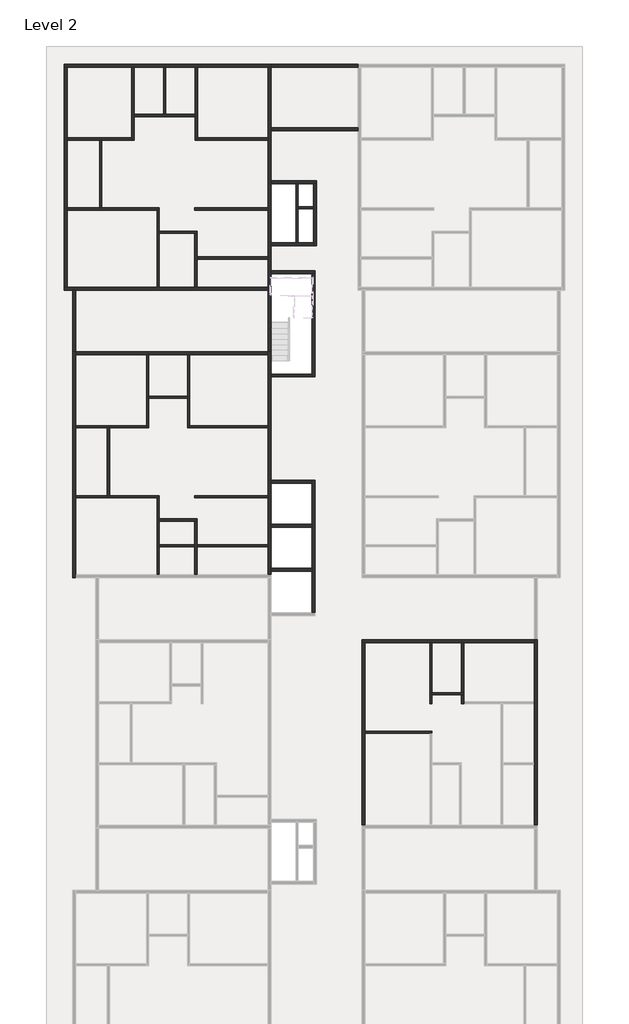
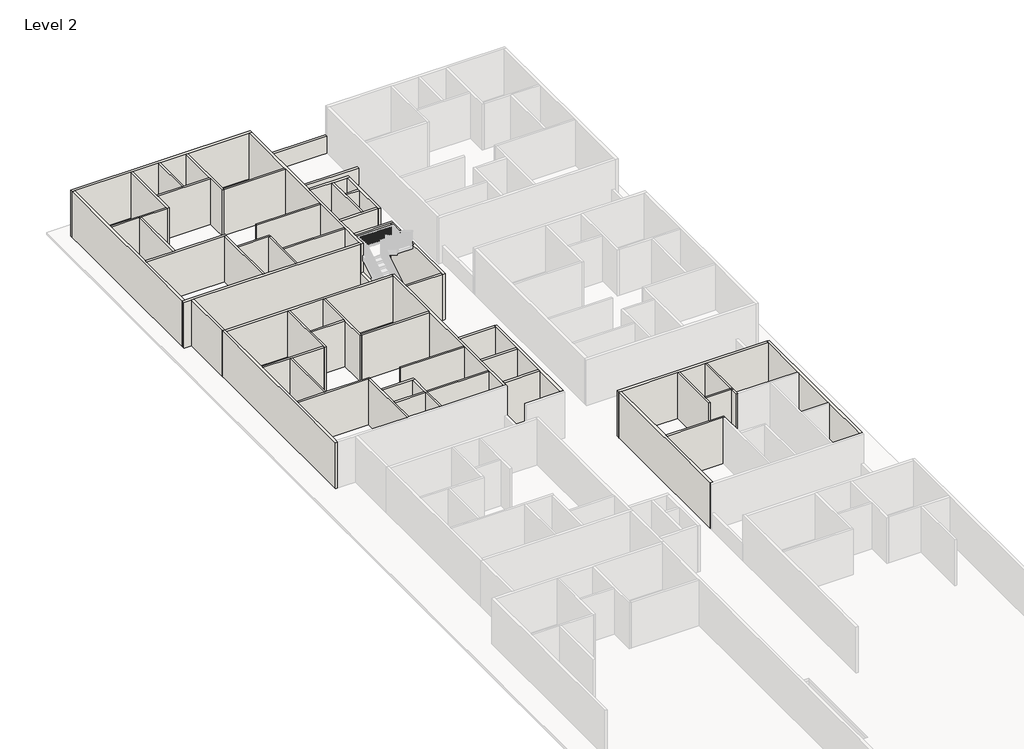
# One storey, part 3 of 8: 57 walls.
"""IFC4 building model written with IfcOpenShell, lengths in millimetres."""

from ifc_helpers import new_model, si_unit, frame, origin, place, context, project, spatial, polyline, outline, extrude, faceted_brep, element, save

model = new_model("IFC4")

# Units and contexts
model_context = context("Model", 3, world=origin())
ifc_project = project(units=[si_unit("LENGTHUNIT", "METRE", prefix="MILLI")], contexts=[model_context])

# Site, building, storey
site = spatial("IfcSite", under=ifc_project)
building = spatial("IfcBuilding", under=site)
storey = spatial("IfcBuildingStorey", under=building, Name="Level 2", Elevation=28282.6172466)

# Walls
placement = place(None, origin())
element("IfcWall", 1, ObjectType="4.5\"", at=placement, inside=storey, context=model_context, shape_type="Brep", body=[
    faceted_brep([(-10818.3415084, 35031.1216096, 28282.6172466), (-10818.3415084, 31373.5216096, 28282.6172466), (-10818.3415084, 31259.2216096, 28282.6172466), (-10818.3415084, 31259.2216096, 31330.6172466), (-10818.3415084, 31373.5216096, 31330.6172466), (-10818.3415084, 35031.1216096, 31330.6172466), (-10704.0415084, 35031.1216096, 28282.6172466), (-10704.0415084, 35031.1216096, 31330.6172466), (-10704.0415084, 32592.7216096, 31330.6172466), (-10704.0415084, 32478.4216096, 31330.6172466), (-10704.0415084, 31259.2216096, 31330.6172466), (-10704.0415084, 31259.2216096, 28282.6172466), (-10704.0415084, 32478.4216096, 28282.6172466), (-10704.0415084, 32592.7216096, 28282.6172466)], [[[0, 1, 2, 3, 4, 5]], [[6, 7, 8, 9, 10, 11, 12, 13]], [[2, 1, 0, 6, 13, 12, 11]], [[0, 5, 7, 6]], [[3, 2, 11, 10]], [[5, 4, 3, 10, 9, 8, 7]]]),
])
element("IfcWall", 2, ObjectType="4.5\"", at=placement, inside=storey, context=model_context, shape_type="Brep", body=[
    faceted_brep([(-10818.3415084, 31373.5216096, 28282.6172466), (-14171.1415084, 31373.5216096, 28282.6172466), (-14171.1415084, 31373.5216096, 31330.6172466), (-10818.3415084, 31373.5216096, 31330.6172466), (-10818.3415084, 31259.2216096, 28282.6172466), (-10818.3415084, 31259.2216096, 31330.6172466), (-12380.4415084, 31259.2216096, 31330.6172466), (-12494.7415084, 31259.2216096, 31330.6172466), (-14171.1415084, 31259.2216096, 31330.6172466), (-14171.1415084, 31259.2216096, 28282.6172466), (-12494.7415084, 31259.2216096, 28282.6172466), (-12380.4415084, 31259.2216096, 28282.6172466)], [[[0, 1, 2, 3]], [[4, 5, 6, 7, 8, 9, 10, 11]], [[1, 0, 4, 11, 10, 9]], [[0, 3, 5, 4]], [[2, 1, 9, 8]], [[3, 2, 8, 7, 6, 5]]]),
])
element("IfcWall", 3, ObjectType="4.5\"", at=placement, inside=storey, context=model_context, shape_type="SweptSolid", body=[
    extrude(outline(polyline([(-12494.7415084, 27754.0216096), (-12494.7415084, 31259.2216096), (-12380.4415084, 31259.2216096), (-12380.4415084, 27754.0216096), (-12494.7415084, 27754.0216096)])), frame((0.0, 0.0, 28282.6172466), z_axis=(0.0, 0.0, 1.0), x_axis=(1.0, 0.0, 0.0)), (0.0, 0.0, 1.0), 3048.0),
])
element("IfcWall", 4, ObjectType="4.5\"", at=placement, inside=storey, context=model_context, shape_type="Brep", body=[
    faceted_brep([(-14171.1415084, 27639.7216096, 28282.6172466), (-9510.2415084, 27639.7216096, 28282.6172466), (-9395.9415084, 27639.7216096, 28282.6172466), (-9395.9415084, 27639.7216096, 31330.6172466), (-9510.2415084, 27639.7216096, 31330.6172466), (-14171.1415084, 27639.7216096, 31330.6172466), (-14171.1415084, 27754.0216096, 28282.6172466), (-14171.1415084, 27754.0216096, 31330.6172466), (-12494.7415084, 27754.0216096, 31330.6172466), (-12380.4415084, 27754.0216096, 31330.6172466), (-9395.9415084, 27754.0216096, 31330.6172466), (-9395.9415084, 27754.0216096, 28282.6172466), (-12380.4415084, 27754.0216096, 28282.6172466), (-12494.7415084, 27754.0216096, 28282.6172466)], [[[0, 1, 2, 3, 4, 5]], [[6, 7, 8, 9, 10, 11, 12, 13]], [[2, 1, 0, 6, 13, 12, 11]], [[0, 5, 7, 6]], [[3, 2, 11, 10]], [[5, 4, 3, 10, 9, 8, 7]]]),
])
element("IfcWall", 5, ObjectType="4.5\"", at=placement, inside=storey, context=model_context, shape_type="Brep", body=[
    faceted_brep([(-9510.2415084, 27639.7216096, 28282.6172466), (-9510.2415084, 23651.9216096, 28282.6172466), (-9510.2415084, 23651.9216096, 31330.6172466), (-9510.2415084, 27639.7216096, 31330.6172466), (-9395.9415084, 27639.7216096, 28282.6172466), (-9395.9415084, 27639.7216096, 31330.6172466), (-9395.9415084, 26547.5216096, 31330.6172466), (-9395.9415084, 26433.2216096, 31330.6172466), (-9395.9415084, 23651.9216096, 31330.6172466), (-9395.9415084, 23651.9216096, 28282.6172466), (-9395.9415084, 26433.2216096, 28282.6172466), (-9395.9415084, 26547.5216096, 28282.6172466)], [[[0, 1, 2, 3]], [[4, 5, 6, 7, 8, 9, 10, 11]], [[1, 0, 4, 11, 10, 9]], [[0, 3, 5, 4]], [[2, 1, 9, 8]], [[3, 2, 8, 7, 6, 5]]]),
])
element("IfcWall", 6, ObjectType="4.5\"", at=placement, inside=storey, context=model_context, shape_type="Brep", body=[
    faceted_brep([(-9395.9415084, 26433.2216096, 28282.6172466), (-7567.1415084, 26433.2216096, 28282.6172466), (-7452.8415084, 26433.2216096, 28282.6172466), (-7452.8415084, 26433.2216096, 31330.6172466), (-7567.1415084, 26433.2216096, 31330.6172466), (-9395.9415084, 26433.2216096, 31330.6172466), (-9395.9415084, 26547.5216096, 28282.6172466), (-9395.9415084, 26547.5216096, 31330.6172466), (-7452.8415084, 26547.5216096, 31330.6172466), (-7452.8415084, 26547.5216096, 28282.6172466)], [[[0, 1, 2, 3, 4, 5]], [[6, 7, 8, 9]], [[2, 1, 0, 6, 9]], [[0, 5, 7, 6]], [[3, 2, 9, 8]], [[5, 4, 3, 8, 7]]]),
])
element("IfcWall", 7, ObjectType="4.5\"", at=placement, inside=storey, context=model_context, shape_type="Brep", body=[
    faceted_brep([(-7567.1415084, 26433.2216096, 28282.6172466), (-7567.1415084, 23651.9216096, 28282.6172466), (-7567.1415084, 23651.9216096, 31330.6172466), (-7567.1415084, 26433.2216096, 31330.6172466), (-7452.8415084, 26433.2216096, 28282.6172466), (-7452.8415084, 26433.2216096, 31330.6172466), (-7452.8415084, 25214.0216096, 31330.6172466), (-7452.8415084, 25099.7216096, 31330.6172466), (-7452.8415084, 23651.9216096, 31330.6172466), (-7452.8415084, 23651.9216096, 28282.6172466), (-7452.8415084, 25099.7216096, 28282.6172466), (-7452.8415084, 25214.0216096, 28282.6172466)], [[[0, 1, 2, 3]], [[4, 5, 6, 7, 8, 9, 10, 11]], [[1, 0, 4, 11, 10, 9]], [[0, 3, 5, 4]], [[2, 1, 9, 8]], [[3, 2, 8, 7, 6, 5]]]),
])
element("IfcWall", 8, ObjectType="4.5\"", at=placement, inside=storey, context=model_context, shape_type="SweptSolid", body=[
    extrude(outline(polyline([(-7452.8415084, 25214.0216096), (-3769.8415084, 25214.0216096), (-3769.8415084, 25099.7216096), (-7452.8415084, 25099.7216096), (-7452.8415084, 25214.0216096)])), frame((0.0, 0.0, 28282.6172466), z_axis=(0.0, 0.0, 1.0), x_axis=(1.0, 0.0, 0.0)), (0.0, 0.0, 1.0), 3048.0),
])
element("IfcWall", 9, ObjectType="4.5\"", at=placement, inside=storey, context=model_context, shape_type="SweptSolid", body=[
    extrude(outline(polyline([(-3769.8415084, 27639.7216096), (-7567.1415084, 27639.7216096), (-7567.1415084, 27754.0216096), (-3769.8415084, 27754.0216096), (-3769.8415084, 27639.7216096)])), frame((0.0, 0.0, 28282.6172466), z_axis=(0.0, 0.0, 1.0), x_axis=(1.0, 0.0, 0.0)), (0.0, 0.0, 1.0), 3048.0),
])
element("IfcWall", 10, ObjectType="4.5\"", at=placement, inside=storey, context=model_context, shape_type="Brep", body=[
    faceted_brep([(-10704.0415084, 32478.4216096, 28282.6172466), (-7541.7415084, 32478.4216096, 28282.6172466), (-7541.7415084, 32478.4216096, 31330.6172466), (-10704.0415084, 32478.4216096, 31330.6172466), (-10704.0415084, 32592.7216096, 28282.6172466), (-10704.0415084, 32592.7216096, 31330.6172466), (-9180.0415084, 32592.7216096, 31330.6172466), (-9065.7415084, 32592.7216096, 31330.6172466), (-7541.7415084, 32592.7216096, 31330.6172466), (-7541.7415084, 32592.7216096, 28282.6172466), (-9065.7415084, 32592.7216096, 28282.6172466), (-9180.0415084, 32592.7216096, 28282.6172466)], [[[0, 1, 2, 3]], [[4, 5, 6, 7, 8, 9, 10, 11]], [[1, 0, 4, 11, 10, 9]], [[0, 3, 5, 4]], [[2, 1, 9, 8]], [[3, 2, 8, 7, 6, 5]]]),
])
element("IfcWall", 11, ObjectType="4.5\"", at=placement, inside=storey, context=model_context, shape_type="SweptSolid", body=[
    extrude(outline(polyline([(-9180.0415084, 32592.7216096), (-9180.0415084, 35031.1216096), (-9065.7415084, 35031.1216096), (-9065.7415084, 32592.7216096), (-9180.0415084, 32592.7216096)])), frame((0.0, 0.0, 28282.6172466), z_axis=(0.0, 0.0, 1.0), x_axis=(1.0, 0.0, 0.0)), (0.0, 0.0, 1.0), 3048.0),
])
element("IfcWall", 12, ObjectType="4.5\"", at=placement, inside=storey, context=model_context, shape_type="Brep", body=[
    faceted_brep([(-7541.7415084, 35031.1216096, 28282.6172466), (-7541.7415084, 32592.7216096, 28282.6172466), (-7541.7415084, 32478.4216096, 28282.6172466), (-7541.7415084, 31259.2216096, 28282.6172466), (-7541.7415084, 31259.2216096, 31330.6172466), (-7541.7415084, 32478.4216096, 31330.6172466), (-7541.7415084, 32592.7216096, 31330.6172466), (-7541.7415084, 35031.1216096, 31330.6172466), (-7427.4415084, 35031.1216096, 28282.6172466), (-7427.4415084, 35031.1216096, 31330.6172466), (-7427.4415084, 31373.5216096, 31330.6172466), (-7427.4415084, 31259.2216096, 31330.6172466), (-7427.4415084, 31259.2216096, 28282.6172466), (-7427.4415084, 31373.5216096, 28282.6172466)], [[[0, 1, 2, 3, 4, 5, 6, 7]], [[8, 9, 10, 11, 12, 13]], [[3, 2, 1, 0, 8, 13, 12]], [[0, 7, 9, 8]], [[4, 3, 12, 11]], [[7, 6, 5, 4, 11, 10, 9]]]),
])
element("IfcWall", 13, ObjectType="4.5\"", at=placement, inside=storey, context=model_context, shape_type="SweptSolid", body=[
    extrude(outline(polyline([(-3769.8415084, 31259.2216096), (-7427.4415084, 31259.2216096), (-7427.4415084, 31373.5216096), (-3769.8415084, 31373.5216096), (-3769.8415084, 31259.2216096)])), frame((0.0, 0.0, 28282.6172466), z_axis=(0.0, 0.0, 1.0), x_axis=(1.0, 0.0, 0.0)), (0.0, 0.0, 1.0), 3048.0),
])
element("IfcWall", 14, ObjectType="4.5\"", at=placement, inside=storey, context=model_context, shape_type="Brep", body=[
    faceted_brep([(-10061.4044854, 20146.7216096, 28282.6172466), (-10061.4044854, 16489.1216096, 28282.6172466), (-10061.4044854, 16374.8216096, 28282.6172466), (-10061.4044854, 16374.8216096, 31330.6172466), (-10061.4044854, 16489.1216096, 31330.6172466), (-10061.4044854, 20146.7216096, 31330.6172466), (-9947.1044854, 20146.7216096, 28282.6172466), (-9947.1044854, 20146.7216096, 31330.6172466), (-9947.1044854, 18013.1216096, 31330.6172466), (-9947.1044854, 17898.8216096, 31330.6172466), (-9947.1044854, 16374.8216096, 31330.6172466), (-9947.1044854, 16374.8216096, 28282.6172466), (-9947.1044854, 17898.8216096, 28282.6172466), (-9947.1044854, 18013.1216096, 28282.6172466)], [[[0, 1, 2, 3, 4, 5]], [[6, 7, 8, 9, 10, 11, 12, 13]], [[2, 1, 0, 6, 13, 12, 11]], [[0, 5, 7, 6]], [[3, 2, 11, 10]], [[5, 4, 3, 10, 9, 8, 7]]]),
])
element("IfcWall", 15, ObjectType="4.5\"", at=placement, inside=storey, context=model_context, shape_type="Brep", body=[
    faceted_brep([(-10061.4044854, 16489.1216096, 28282.6172466), (-13719.0044854, 16489.1216096, 28282.6172466), (-13719.0044854, 16489.1216096, 31330.6172466), (-10061.4044854, 16489.1216096, 31330.6172466), (-10061.4044854, 16374.8216096, 28282.6172466), (-10061.4044854, 16374.8216096, 31330.6172466), (-11980.3915084, 16374.8216096, 31330.6172466), (-12094.6915084, 16374.8216096, 31330.6172466), (-13719.0044854, 16374.8216096, 31330.6172466), (-13719.0044854, 16374.8216096, 28282.6172466), (-12094.6915084, 16374.8216096, 28282.6172466), (-11980.3915084, 16374.8216096, 28282.6172466)], [[[0, 1, 2, 3]], [[4, 5, 6, 7, 8, 9, 10, 11]], [[1, 0, 4, 11, 10, 9]], [[0, 3, 5, 4]], [[2, 1, 9, 8]], [[3, 2, 8, 7, 6, 5]]]),
])
element("IfcWall", 16, ObjectType="4.5\"", at=placement, inside=storey, context=model_context, shape_type="SweptSolid", body=[
    extrude(outline(polyline([(-7940.5044854, 17898.8216096), (-9947.1044854, 17898.8216096), (-9947.1044854, 18013.1216096), (-7940.5044854, 18013.1216096), (-7940.5044854, 17898.8216096)])), frame((0.0, 0.0, 28282.6172466), z_axis=(0.0, 0.0, 1.0), x_axis=(1.0, 0.0, 0.0)), (0.0, 0.0, 1.0), 3048.0),
])
element("IfcWall", 17, ObjectType="4.5\"", at=placement, inside=storey, context=model_context, shape_type="Brep", body=[
    faceted_brep([(-7940.5044854, 20146.7216096, 28282.6172466), (-7940.5044854, 18013.1216096, 28282.6172466), (-7940.5044854, 17898.8216096, 28282.6172466), (-7940.5044854, 16374.8216096, 28282.6172466), (-7940.5044854, 16374.8216096, 31330.6172466), (-7940.5044854, 17898.8216096, 31330.6172466), (-7940.5044854, 18013.1216096, 31330.6172466), (-7940.5044854, 20146.7216096, 31330.6172466), (-7826.2044854, 20146.7216096, 28282.6172466), (-7826.2044854, 20146.7216096, 31330.6172466), (-7826.2044854, 16489.1216096, 31330.6172466), (-7826.2044854, 16374.8216096, 31330.6172466), (-7826.2044854, 16374.8216096, 28282.6172466), (-7826.2044854, 16489.1216096, 28282.6172466)], [[[0, 1, 2, 3, 4, 5, 6, 7]], [[8, 9, 10, 11, 12, 13]], [[3, 2, 1, 0, 8, 13, 12]], [[0, 7, 9, 8]], [[4, 3, 12, 11]], [[7, 6, 5, 4, 11, 10, 9]]]),
])
element("IfcWall", 18, ObjectType="4.5\"", at=placement, inside=storey, context=model_context, shape_type="SweptSolid", body=[
    extrude(outline(polyline([(-3769.8415084, 16374.8216096), (-7826.2044854, 16374.8216096), (-7826.2044854, 16489.1216096), (-3769.8415084, 16489.1216096), (-3769.8415084, 16374.8216096)])), frame((0.0, 0.0, 28282.6172466), z_axis=(0.0, 0.0, 1.0), x_axis=(1.0, 0.0, 0.0)), (0.0, 0.0, 1.0), 3048.0),
])
element("IfcWall", 19, ObjectType="4.5\"", at=placement, inside=storey, context=model_context, shape_type="SweptSolid", body=[
    extrude(outline(polyline([(-12094.6915084, 12869.6216096), (-12094.6915084, 16374.8216096), (-11980.3915084, 16374.8216096), (-11980.3915084, 12869.6216096), (-12094.6915084, 12869.6216096)])), frame((0.0, 0.0, 28282.6172466), z_axis=(0.0, 0.0, 1.0), x_axis=(1.0, 0.0, 0.0)), (0.0, 0.0, 1.0), 3048.0),
])
element("IfcWall", 20, ObjectType="4.5\"", at=placement, inside=storey, context=model_context, shape_type="Brep", body=[
    faceted_brep([(-13719.0044854, 12755.3216096, 28282.6172466), (-9510.2415084, 12755.3216096, 28282.6172466), (-9395.9415084, 12755.3216096, 28282.6172466), (-9395.9415084, 12755.3216096, 31330.6172466), (-9510.2415084, 12755.3216096, 31330.6172466), (-13719.0044854, 12755.3216096, 31330.6172466), (-13719.0044854, 12869.6216096, 28282.6172466), (-13719.0044854, 12869.6216096, 31330.6172466), (-12094.6915084, 12869.6216096, 31330.6172466), (-11980.3915084, 12869.6216096, 31330.6172466), (-9395.9415084, 12869.6216096, 31330.6172466), (-9395.9415084, 12869.6216096, 28282.6172466), (-11980.3915084, 12869.6216096, 28282.6172466), (-12094.6915084, 12869.6216096, 28282.6172466)], [[[0, 1, 2, 3, 4, 5]], [[6, 7, 8, 9, 10, 11, 12, 13]], [[2, 1, 0, 6, 13, 12, 11]], [[0, 5, 7, 6]], [[3, 2, 11, 10]], [[5, 4, 3, 10, 9, 8, 7]]]),
])
element("IfcWall", 21, ObjectType="4.5\"", at=placement, inside=storey, context=model_context, shape_type="Brep", body=[
    faceted_brep([(-9510.2415084, 12755.3216096, 28282.6172466), (-9510.2415084, 8767.5216096, 28282.6172466), (-9510.2415084, 8767.5216096, 31330.6172466), (-9510.2415084, 12755.3216096, 31330.6172466), (-9395.9415084, 12755.3216096, 28282.6172466), (-9395.9415084, 12755.3216096, 31330.6172466), (-9395.9415084, 11663.1216096, 31330.6172466), (-9395.9415084, 11548.8216096, 31330.6172466), (-9395.9415084, 10329.6216096, 31330.6172466), (-9395.9415084, 10215.3216096, 31330.6172466), (-9395.9415084, 8767.5216096, 31330.6172466), (-9395.9415084, 8767.5216096, 28282.6172466), (-9395.9415084, 10215.3216096, 28282.6172466), (-9395.9415084, 10329.6216096, 28282.6172466), (-9395.9415084, 11548.8216096, 28282.6172466), (-9395.9415084, 11663.1216096, 28282.6172466)], [[[0, 1, 2, 3]], [[4, 5, 6, 7, 8, 9, 10, 11, 12, 13, 14, 15]], [[1, 0, 4, 15, 14, 13, 12, 11]], [[0, 3, 5, 4]], [[2, 1, 11, 10]], [[3, 2, 10, 9, 8, 7, 6, 5]]]),
])
element("IfcWall", 22, ObjectType="4.5\"", at=placement, inside=storey, context=model_context, shape_type="SweptSolid", body=[
    extrude(outline(polyline([(-7567.1415084, 10215.3216096), (-9395.9415084, 10215.3216096), (-9395.9415084, 10329.6216096), (-7567.1415084, 10329.6216096), (-7567.1415084, 10215.3216096)])), frame((0.0, 0.0, 28282.6172466), z_axis=(0.0, 0.0, 1.0), x_axis=(1.0, 0.0, 0.0)), (0.0, 0.0, 1.0), 3048.0),
])
element("IfcWall", 23, ObjectType="4.5\"", at=placement, inside=storey, context=model_context, shape_type="Brep", body=[
    faceted_brep([(-9395.9415084, 11548.8216096, 28282.6172466), (-7567.1415084, 11548.8216096, 28282.6172466), (-7452.8415084, 11548.8216096, 28282.6172466), (-7452.8415084, 11548.8216096, 31330.6172466), (-7567.1415084, 11548.8216096, 31330.6172466), (-9395.9415084, 11548.8216096, 31330.6172466), (-9395.9415084, 11663.1216096, 28282.6172466), (-9395.9415084, 11663.1216096, 31330.6172466), (-7452.8415084, 11663.1216096, 31330.6172466), (-7452.8415084, 11663.1216096, 28282.6172466)], [[[0, 1, 2, 3, 4, 5]], [[6, 7, 8, 9]], [[2, 1, 0, 6, 9]], [[0, 5, 7, 6]], [[3, 2, 9, 8]], [[5, 4, 3, 8, 7]]]),
])
element("IfcWall", 24, ObjectType="4.5\"", at=placement, inside=storey, context=model_context, shape_type="Brep", body=[
    faceted_brep([(-7567.1415084, 11548.8216096, 28282.6172466), (-7567.1415084, 10329.6216096, 28282.6172466), (-7567.1415084, 10215.3216096, 28282.6172466), (-7567.1415084, 8767.5216096, 28282.6172466), (-7567.1415084, 8767.5216096, 31330.6172466), (-7567.1415084, 10215.3216096, 31330.6172466), (-7567.1415084, 10329.6216096, 31330.6172466), (-7567.1415084, 11548.8216096, 31330.6172466), (-7452.8415084, 11548.8216096, 28282.6172466), (-7452.8415084, 11548.8216096, 31330.6172466), (-7452.8415084, 10329.6216096, 31330.6172466), (-7452.8415084, 10215.3216096, 31330.6172466), (-7452.8415084, 8767.5216096, 31330.6172466), (-7452.8415084, 8767.5216096, 28282.6172466), (-7452.8415084, 10215.3216096, 28282.6172466), (-7452.8415084, 10329.6216096, 28282.6172466)], [[[0, 1, 2, 3, 4, 5, 6, 7]], [[8, 9, 10, 11, 12, 13, 14, 15]], [[3, 2, 1, 0, 8, 15, 14, 13]], [[0, 7, 9, 8]], [[4, 3, 13, 12]], [[7, 6, 5, 4, 12, 11, 10, 9]]]),
])
element("IfcWall", 25, ObjectType="4.5\"", at=placement, inside=storey, context=model_context, shape_type="SweptSolid", body=[
    extrude(outline(polyline([(-3769.8415084, 10215.3216096), (-7452.8415084, 10215.3216096), (-7452.8415084, 10329.6216096), (-3769.8415084, 10329.6216096), (-3769.8415084, 10215.3216096)])), frame((0.0, 0.0, 28282.6172466), z_axis=(0.0, 0.0, 1.0), x_axis=(1.0, 0.0, 0.0)), (0.0, 0.0, 1.0), 3048.0),
])
element("IfcWall", 26, ObjectType="4.5\"", at=placement, inside=storey, context=model_context, shape_type="SweptSolid", body=[
    extrude(outline(polyline([(-3769.8415084, 12755.3216096), (-7567.1415084, 12755.3216096), (-7567.1415084, 12869.6216096), (-3769.8415084, 12869.6216096), (-3769.8415084, 12755.3216096)])), frame((0.0, 0.0, 28282.6172466), z_axis=(0.0, 0.0, 1.0), x_axis=(1.0, 0.0, 0.0)), (0.0, 0.0, 1.0), 3048.0),
])
element("IfcWall", 27, ObjectType="4.5\"", at=placement, inside=storey, context=model_context, shape_type="Brep", body=[
    faceted_brep([(1259.3584916, 572.7745083, 28282.6172466), (4610.8714687, 572.7745083, 28282.6172466), (4725.1714687, 572.7745083, 28282.6172466), (4725.1714687, 572.7745083, 31330.6172466), (4610.8714687, 572.7745083, 31330.6172466), (1259.3584916, 572.7745083, 31330.6172466), (1259.3584916, 687.0745083, 28282.6172466), (1259.3584916, 687.0745083, 31330.6172466), (4725.1714687, 687.0745083, 31330.6172466), (4725.1714687, 687.0745083, 28282.6172466)], [[[0, 1, 2, 3, 4, 5]], [[6, 7, 8, 9]], [[2, 1, 0, 6, 9]], [[0, 5, 7, 6]], [[3, 2, 9, 8]], [[5, 4, 3, 8, 7]]]),
])
element("IfcWall", 28, ObjectType="4.5\"", at=placement, inside=storey, context=model_context, shape_type="Brep", body=[
    faceted_brep([(4610.8714687, 5262.3216096, 28282.6172466), (4610.8714687, 2100.0216096, 28282.6172466), (4610.8714687, 2100.0216096, 31330.6172466), (4610.8714687, 5262.3216096, 31330.6172466), (4725.1714687, 5262.3216096, 28282.6172466), (4725.1714687, 5262.3216096, 31330.6172466), (4725.1714687, 2671.5216096, 31330.6172466), (4725.1714687, 2557.2216096, 31330.6172466), (4725.1714687, 2100.0216096, 31330.6172466), (4725.1714687, 2100.0216096, 28282.6172466), (4725.1714687, 2557.2216096, 28282.6172466), (4725.1714687, 2671.5216096, 28282.6172466)], [[[0, 1, 2, 3]], [[4, 5, 6, 7, 8, 9, 10, 11]], [[1, 0, 4, 11, 10, 9]], [[2, 1, 9, 8]], [[0, 3, 5, 4]], [[3, 2, 8, 7, 6, 5]]]),
])
element("IfcWall", 29, ObjectType="4.5\"", at=placement, inside=storey, context=model_context, shape_type="Brep", body=[
    faceted_brep([(4725.1714687, 2557.2216096, 28282.6172466), (6249.1714687, 2557.2216096, 28282.6172466), (6363.4714687, 2557.2216096, 28282.6172466), (6363.4714687, 2557.2216096, 31330.6172466), (6249.1714687, 2557.2216096, 31330.6172466), (4725.1714687, 2557.2216096, 31330.6172466), (4725.1714687, 2671.5216096, 28282.6172466), (4725.1714687, 2671.5216096, 31330.6172466), (6249.1714687, 2671.5216096, 31330.6172466), (6363.4714687, 2671.5216096, 31330.6172466), (6363.4714687, 2671.5216096, 28282.6172466), (6249.1714687, 2671.5216096, 28282.6172466)], [[[0, 1, 2, 3, 4, 5]], [[6, 7, 8, 9, 10, 11]], [[2, 1, 0, 6, 11, 10]], [[0, 5, 7, 6]], [[3, 2, 10, 9]], [[5, 4, 3, 9, 8, 7]]]),
])
element("IfcWall", 30, ObjectType="4.5\"", at=placement, inside=storey, context=model_context, shape_type="SweptSolid", body=[
    extrude(outline(polyline([(6363.4714687, 5262.3216096), (6363.4714687, 2671.5216096), (6249.1714687, 2671.5216096), (6249.1714687, 5262.3216096), (6363.4714687, 5262.3216096)])), frame((0.0, 0.0, 28282.6172466), z_axis=(0.0, 0.0, 1.0), x_axis=(1.0, 0.0, 0.0)), (0.0, 0.0, 1.0), 3048.0),
])
element("IfcWall", 31, ObjectType="4.5\"", at=placement, inside=storey, context=model_context, shape_type="Brep", body=[
    faceted_brep([(6249.1714687, 2557.2216096, 28282.6172466), (6249.1714687, 2100.0216096, 28282.6172466), (6249.1714687, 2100.0216096, 31330.6172466), (6249.1714687, 2557.2216096, 31330.6172466), (6363.4714687, 2557.2216096, 28282.6172466), (6363.4714687, 2557.2216096, 31330.6172466), (6363.4714687, 2214.3216096, 31330.6172466), (6363.4714687, 2100.0216096, 31330.6172466), (6363.4714687, 2100.0216096, 28282.6172466), (6363.4714687, 2214.3216096, 28282.6172466)], [[[0, 1, 2, 3]], [[4, 5, 6, 7, 8, 9]], [[1, 0, 4, 9, 8]], [[0, 3, 5, 4]], [[2, 1, 8, 7]], [[3, 2, 7, 6, 5]]]),
])
element("IfcWall", 32, ObjectType="4.5\"", at=placement, inside=storey, context=model_context, shape_type="Brep", body=[
    faceted_brep([(-2321.9738684, 29000.0900967, 28282.6172466), (-2321.9738684, 25952.0900967, 28282.6172466), (-2321.9738684, 25952.0900967, 31330.6172466), (-2321.9738684, 29000.0900967, 31330.6172466), (-2207.6738684, 29000.0900967, 28282.6172466), (-2207.6738684, 29000.0900967, 31330.6172466), (-2207.6738684, 27820.8172885, 31330.6172466), (-2207.6738684, 27706.5172885, 31330.6172466), (-2207.6738684, 25952.0900967, 31330.6172466), (-2207.6738684, 25952.0900967, 28282.6172466), (-2207.6738684, 27706.5172885, 28282.6172466), (-2207.6738684, 27820.8172885, 28282.6172466)], [[[0, 1, 2, 3]], [[4, 5, 6, 7, 8, 9, 10, 11]], [[1, 0, 4, 11, 10, 9]], [[3, 2, 8, 7, 6, 5]], [[0, 3, 5, 4]], [[2, 1, 9, 8]]]),
])
element("IfcWall", 33, ObjectType="4.5\"", at=placement, inside=storey, context=model_context, shape_type="SweptSolid", body=[
    extrude(outline(polyline([(-2207.6738684, 27820.8172885), (-1407.6415084, 27820.8172885), (-1407.6415084, 27706.5172885), (-2207.6738684, 27706.5172885), (-2207.6738684, 27820.8172885)])), frame((0.0, 0.0, 28282.6172466), z_axis=(0.0, 0.0, 1.0), x_axis=(1.0, 0.0, 0.0)), (0.0, 0.0, 1.0), 3048.0),
])
element("IfcWall", 34, ObjectType="6\"", at=placement, inside=storey, context=model_context, shape_type="Brep", body=[
    faceted_brep([(-14323.5415084, 35031.1216096, 28282.6172466), (-14171.1415084, 35031.1216096, 28282.6172466), (-10818.3415084, 35031.1216096, 28282.6172466), (-10704.0415084, 35031.1216096, 28282.6172466), (-9180.0415084, 35031.1216096, 28282.6172466), (-9065.7415084, 35031.1216096, 28282.6172466), (-7541.7415084, 35031.1216096, 28282.6172466), (-7427.4415084, 35031.1216096, 28282.6172466), (-3769.8415084, 35031.1216096, 28282.6172466), (-3617.4415084, 35031.1216096, 28282.6172466), (-3617.4415084, 35031.1216096, 31330.6172466), (-3769.8415084, 35031.1216096, 31330.6172466), (-7427.4415084, 35031.1216096, 31330.6172466), (-7541.7415084, 35031.1216096, 31330.6172466), (-9065.7415084, 35031.1216096, 31330.6172466), (-9180.0415084, 35031.1216096, 31330.6172466), (-10704.0415084, 35031.1216096, 31330.6172466), (-10818.3415084, 35031.1216096, 31330.6172466), (-14171.1415084, 35031.1216096, 31330.6172466), (-14323.5415084, 35031.1216096, 31330.6172466), (-14323.5415084, 35183.5216096, 28282.6172466), (-14323.5415084, 35183.5216096, 31330.6172466), (-3617.4415084, 35183.5216096, 31330.6172466), (-3617.4415084, 35183.5216096, 28282.6172466)], [[[0, 1, 2, 3, 4, 5, 6, 7, 8, 9, 10, 11, 12, 13, 14, 15, 16, 17, 18, 19]], [[20, 21, 22, 23]], [[9, 8, 7, 6, 5, 4, 3, 2, 1, 0, 20, 23]], [[0, 19, 21, 20]], [[9, 23, 22, 10]], [[19, 18, 17, 16, 15, 14, 13, 12, 11, 10, 22, 21]]]),
])
element("IfcWall", 35, ObjectType="6\"", at=placement, inside=storey, context=model_context, shape_type="Brep", body=[
    faceted_brep([(-3769.8415084, 35031.1216096, 31330.6172466), (-3769.8415084, 35031.1216096, 28282.6172466), (-3769.8415084, 31373.5216096, 28282.6172466), (-3769.8415084, 31259.2216096, 28282.6172466), (-3769.8415084, 27754.0216096, 28282.6172466), (-3769.8415084, 27639.7216096, 28282.6172466), (-3769.8415084, 25214.0216096, 28282.6172466), (-3769.8415084, 25099.7216096, 28282.6172466), (-3769.8415084, 23651.9216096, 28282.6172466), (-3769.8415084, 23499.5216096, 28282.6172466), (-3769.8415084, 23499.5216096, 31330.6172466), (-3769.8415084, 23651.9216096, 31330.6172466), (-3769.8415084, 25099.7216096, 31330.6172466), (-3769.8415084, 25214.0216096, 31330.6172466), (-3769.8415084, 27639.7216096, 31330.6172466), (-3769.8415084, 27754.0216096, 31330.6172466), (-3769.8415084, 31259.2216096, 31330.6172466), (-3769.8415084, 31373.5216096, 31330.6172466), (-3617.4415084, 35031.1216096, 28282.6172466), (-3617.4415084, 35031.1216096, 31330.6172466), (-3617.4415084, 29152.4900967, 31330.6172466), (-3617.4415084, 29000.0900967, 31330.6172466), (-3617.4415084, 25952.0900967, 31330.6172466), (-3617.4415084, 25799.6900967, 31330.6172466), (-3617.4415084, 24490.1216096, 31330.6172466), (-3617.4415084, 24337.7216096, 31330.6172466), (-3617.4415084, 23499.5216096, 31330.6172466), (-3617.4415084, 23499.5216096, 28282.6172466), (-3617.4415084, 24337.7216096, 28282.6172466), (-3617.4415084, 24490.1216096, 28282.6172466), (-3617.4415084, 25799.6900967, 28282.6172466), (-3617.4415084, 25952.0900967, 28282.6172466), (-3617.4415084, 29000.0900967, 28282.6172466), (-3617.4415084, 29152.4900967, 28282.6172466), (-3617.4415084, 31744.9197155, 28282.6172466), (-3617.4415084, 31897.3197155, 28282.6172466)], [[[0, 1, 2, 3, 4, 5, 6, 7, 8, 9, 10, 11, 12, 13, 14, 15, 16, 17]], [[18, 19, 20, 21, 22, 23, 24, 25, 26, 27, 28, 29, 30, 31, 32, 33, 34, 35]], [[9, 8, 7, 6, 5, 4, 3, 2, 1, 18, 35, 34, 33, 32, 31, 30, 29, 28, 27]], [[0, 19, 18, 1]], [[9, 27, 26, 10]], [[0, 17, 16, 15, 14, 13, 12, 11, 10, 26, 25, 24, 23, 22, 21, 20, 19]]]),
])
element("IfcWall", 36, ObjectType="6\"", at=placement, inside=storey, context=model_context, shape_type="Brep", body=[
    faceted_brep([(-3769.8415084, 23651.9216096, 31330.6172466), (-3769.8415084, 23651.9216096, 28282.6172466), (-7452.8415084, 23651.9216096, 28282.6172466), (-7567.1415084, 23651.9216096, 28282.6172466), (-9395.9415084, 23651.9216096, 28282.6172466), (-9510.2415084, 23651.9216096, 28282.6172466), (-14171.1415084, 23651.9216096, 28282.6172466), (-14323.5415084, 23651.9216096, 28282.6172466), (-14323.5415084, 23651.9216096, 31330.6172466), (-14171.1415084, 23651.9216096, 31330.6172466), (-9510.2415084, 23651.9216096, 31330.6172466), (-9395.9415084, 23651.9216096, 31330.6172466), (-7567.1415084, 23651.9216096, 31330.6172466), (-7452.8415084, 23651.9216096, 31330.6172466), (-3769.8415084, 23499.5216096, 28282.6172466), (-3769.8415084, 23499.5216096, 31330.6172466), (-13719.0044854, 23499.5216096, 31330.6172466), (-13871.4044854, 23499.5216096, 31330.6172466), (-14323.5415084, 23499.5216096, 31330.6172466), (-14323.5415084, 23499.5216096, 28282.6172466), (-13871.4044854, 23499.5216096, 28282.6172466), (-13719.0044854, 23499.5216096, 28282.6172466)], [[[0, 1, 2, 3, 4, 5, 6, 7, 8, 9, 10, 11, 12, 13]], [[14, 15, 16, 17, 18, 19, 20, 21]], [[7, 6, 5, 4, 3, 2, 1, 14, 21, 20, 19]], [[8, 7, 19, 18]], [[0, 15, 14, 1]], [[0, 13, 12, 11, 10, 9, 8, 18, 17, 16, 15]]]),
])
element("IfcWall", 37, ObjectType="6\"", at=placement, inside=storey, context=model_context, shape_type="Brep", body=[
    faceted_brep([(-14171.1415084, 23651.9216096, 28282.6172466), (-14171.1415084, 27639.7216096, 28282.6172466), (-14171.1415084, 27754.0216096, 28282.6172466), (-14171.1415084, 31259.2216096, 28282.6172466), (-14171.1415084, 31373.5216096, 28282.6172466), (-14171.1415084, 35031.1216096, 28282.6172466), (-14171.1415084, 35031.1216096, 31330.6172466), (-14171.1415084, 31373.5216096, 31330.6172466), (-14171.1415084, 31259.2216096, 31330.6172466), (-14171.1415084, 27754.0216096, 31330.6172466), (-14171.1415084, 27639.7216096, 31330.6172466), (-14171.1415084, 23651.9216096, 31330.6172466), (-14323.5415084, 23651.9216096, 28282.6172466), (-14323.5415084, 23651.9216096, 31330.6172466), (-14323.5415084, 35031.1216096, 31330.6172466), (-14323.5415084, 35031.1216096, 28282.6172466)], [[[0, 1, 2, 3, 4, 5, 6, 7, 8, 9, 10, 11]], [[12, 13, 14, 15]], [[5, 4, 3, 2, 1, 0, 12, 15]], [[6, 5, 15, 14]], [[0, 11, 13, 12]], [[11, 10, 9, 8, 7, 6, 14, 13]]]),
])
element("IfcWall", 38, ObjectType="6\"", at=placement, inside=storey, context=model_context, shape_type="Brep", body=[
    faceted_brep([(-13871.4044854, 20299.1216096, 28282.6172466), (-13871.4044854, 8615.1216096, 28282.6172466), (-13871.4044854, 8615.1216096, 31330.6172466), (-13871.4044854, 20299.1216096, 31330.6172466), (-13719.0044854, 20299.1216096, 28282.6172466), (-13719.0044854, 20299.1216096, 31330.6172466), (-13719.0044854, 20146.7216096, 31330.6172466), (-13719.0044854, 16489.1216096, 31330.6172466), (-13719.0044854, 16374.8216096, 31330.6172466), (-13719.0044854, 12869.6216096, 31330.6172466), (-13719.0044854, 12755.3216096, 31330.6172466), (-13719.0044854, 8767.5216096, 31330.6172466), (-13719.0044854, 8615.1216096, 31330.6172466), (-13719.0044854, 8615.1216096, 28282.6172466), (-13719.0044854, 8767.5216096, 28282.6172466), (-13719.0044854, 12755.3216096, 28282.6172466), (-13719.0044854, 12869.6216096, 28282.6172466), (-13719.0044854, 16374.8216096, 28282.6172466), (-13719.0044854, 16489.1216096, 28282.6172466), (-13719.0044854, 20146.7216096, 28282.6172466)], [[[0, 1, 2, 3]], [[4, 5, 6, 7, 8, 9, 10, 11, 12, 13, 14, 15, 16, 17, 18, 19]], [[1, 0, 4, 19, 18, 17, 16, 15, 14, 13]], [[2, 1, 13, 12]], [[0, 3, 5, 4]], [[3, 2, 12, 11, 10, 9, 8, 7, 6, 5]]]),
])
element("IfcWall", 39, ObjectType="6\"", at=placement, inside=storey, context=model_context, shape_type="Brep", body=[
    faceted_brep([(-3617.4415084, 8767.5216096, 31330.6172466), (-3617.4415084, 8767.5216096, 28282.6172466), (-3617.4415084, 8945.2303368, 28282.6172466), (-3617.4415084, 9097.6303368, 28282.6172466), (-3617.4415084, 11231.2303368, 28282.6172466), (-3617.4415084, 11383.6303368, 28282.6172466), (-3617.4415084, 13517.2303368, 28282.6172466), (-3617.4415084, 13669.6303368, 28282.6172466), (-3617.4415084, 19003.7216096, 28282.6172466), (-3617.4415084, 19156.1216096, 28282.6172466), (-3617.4415084, 20299.1216096, 28282.6172466), (-3617.4415084, 20299.1216096, 31330.6172466), (-3617.4415084, 19156.1216096, 31330.6172466), (-3617.4415084, 19003.7216096, 31330.6172466), (-3617.4415084, 13669.6303368, 31330.6172466), (-3617.4415084, 13517.2303368, 31330.6172466), (-3617.4415084, 11383.6303368, 31330.6172466), (-3617.4415084, 11231.2303368, 31330.6172466), (-3617.4415084, 9097.6303368, 31330.6172466), (-3617.4415084, 8945.2303368, 31330.6172466), (-3769.8415084, 8767.5216096, 28282.6172466), (-3769.8415084, 8767.5216096, 31330.6172466), (-3769.8415084, 10215.3216096, 31330.6172466), (-3769.8415084, 10329.6216096, 31330.6172466), (-3769.8415084, 12755.3216096, 31330.6172466), (-3769.8415084, 12869.6216096, 31330.6172466), (-3769.8415084, 16374.8216096, 31330.6172466), (-3769.8415084, 16489.1216096, 31330.6172466), (-3769.8415084, 20146.7216096, 31330.6172466), (-3769.8415084, 20299.1216096, 31330.6172466), (-3769.8415084, 20299.1216096, 28282.6172466), (-3769.8415084, 20146.7216096, 28282.6172466), (-3769.8415084, 16489.1216096, 28282.6172466), (-3769.8415084, 16374.8216096, 28282.6172466), (-3769.8415084, 12869.6216096, 28282.6172466), (-3769.8415084, 12755.3216096, 28282.6172466), (-3769.8415084, 10329.6216096, 28282.6172466), (-3769.8415084, 10215.3216096, 28282.6172466)], [[[0, 1, 2, 3, 4, 5, 6, 7, 8, 9, 10, 11, 12, 13, 14, 15, 16, 17, 18, 19]], [[20, 21, 22, 23, 24, 25, 26, 27, 28, 29, 30, 31, 32, 33, 34, 35, 36, 37]], [[10, 9, 8, 7, 6, 5, 4, 3, 2, 1, 20, 37, 36, 35, 34, 33, 32, 31, 30]], [[10, 30, 29, 11]], [[0, 21, 20, 1]], [[0, 19, 18, 17, 16, 15, 14, 13, 12, 11, 29, 28, 27, 26, 25, 24, 23, 22, 21]]]),
])
element("IfcWall", 40, ObjectType="6\"", at=placement, inside=storey, context=model_context, shape_type="Brep", body=[
    faceted_brep([(-3769.8415084, 20299.1216096, 31330.6172466), (-3769.8415084, 20299.1216096, 28282.6172466), (-13719.0044854, 20299.1216096, 28282.6172466), (-13719.0044854, 20299.1216096, 31330.6172466), (-3769.8415084, 20146.7216096, 28282.6172466), (-3769.8415084, 20146.7216096, 31330.6172466), (-7826.2044854, 20146.7216096, 31330.6172466), (-7940.5044854, 20146.7216096, 31330.6172466), (-9947.1044854, 20146.7216096, 31330.6172466), (-10061.4044854, 20146.7216096, 31330.6172466), (-13719.0044854, 20146.7216096, 31330.6172466), (-13719.0044854, 20146.7216096, 28282.6172466), (-10061.4044854, 20146.7216096, 28282.6172466), (-9947.1044854, 20146.7216096, 28282.6172466), (-7940.5044854, 20146.7216096, 28282.6172466), (-7826.2044854, 20146.7216096, 28282.6172466)], [[[0, 1, 2, 3]], [[4, 5, 6, 7, 8, 9, 10, 11, 12, 13, 14, 15]], [[2, 1, 4, 15, 14, 13, 12, 11]], [[3, 2, 11, 10]], [[0, 5, 4, 1]], [[0, 3, 10, 9, 8, 7, 6, 5]]]),
])
element("IfcWall", 41, ObjectType="6\"", at=placement, inside=storey, context=model_context, shape_type="Brep", body=[
    faceted_brep([(10173.4714687, -4185.9344126, 31330.6172466), (10173.4714687, -4185.9344126, 28282.6172466), (10173.4714687, 5414.7216096, 28282.6172466), (10173.4714687, 5414.7216096, 31330.6172466), (10021.0714687, -4185.9344126, 28282.6172466), (10021.0714687, -4185.9344126, 31330.6172466), (10021.0714687, -1061.7344126, 31330.6172466), (10021.0714687, -947.4344126, 31330.6172466), (10021.0714687, 2100.0216096, 31330.6172466), (10021.0714687, 2214.3216096, 31330.6172466), (10021.0714687, 5262.3216096, 31330.6172466), (10021.0714687, 5414.7216096, 31330.6172466), (10021.0714687, 5414.7216096, 28282.6172466), (10021.0714687, 5262.3216096, 28282.6172466), (10021.0714687, 2214.3216096, 28282.6172466), (10021.0714687, 2100.0216096, 28282.6172466), (10021.0714687, -947.4344126, 28282.6172466), (10021.0714687, -1061.7344126, 28282.6172466)], [[[0, 1, 2, 3]], [[4, 5, 6, 7, 8, 9, 10, 11, 12, 13, 14, 15, 16, 17]], [[2, 1, 4, 17, 16, 15, 14, 13, 12]], [[2, 12, 11, 3]], [[0, 5, 4, 1]], [[0, 3, 11, 10, 9, 8, 7, 6, 5]]]),
])
element("IfcWall", 42, ObjectType="6\"", at=placement, inside=storey, context=model_context, shape_type="Brep", body=[
    faceted_brep([(10021.0714687, 5414.7216096, 31330.6172466), (10021.0714687, 5414.7216096, 28282.6172466), (1106.9584916, 5414.7216096, 28282.6172466), (1106.9584916, 5414.7216096, 31330.6172466), (10021.0714687, 5262.3216096, 28282.6172466), (10021.0714687, 5262.3216096, 31330.6172466), (6363.4714687, 5262.3216096, 31330.6172466), (6249.1714687, 5262.3216096, 31330.6172466), (4725.1714687, 5262.3216096, 31330.6172466), (4610.8714687, 5262.3216096, 31330.6172466), (1259.3584916, 5262.3216096, 31330.6172466), (1106.9584916, 5262.3216096, 31330.6172466), (1106.9584916, 5262.3216096, 28282.6172466), (1259.3584916, 5262.3216096, 28282.6172466), (4610.8714687, 5262.3216096, 28282.6172466), (4725.1714687, 5262.3216096, 28282.6172466), (6249.1714687, 5262.3216096, 28282.6172466), (6363.4714687, 5262.3216096, 28282.6172466)], [[[0, 1, 2, 3]], [[4, 5, 6, 7, 8, 9, 10, 11, 12, 13, 14, 15, 16, 17]], [[2, 1, 4, 17, 16, 15, 14, 13, 12]], [[3, 2, 12, 11]], [[0, 5, 4, 1]], [[0, 3, 11, 10, 9, 8, 7, 6, 5]]]),
])
element("IfcWall", 43, ObjectType="6\"", at=placement, inside=storey, context=model_context, shape_type="Brep", body=[
    faceted_brep([(1106.9584916, 5262.3216096, 28282.6172466), (1106.9584916, -4185.9344126, 28282.6172466), (1106.9584916, -4185.9344126, 31330.6172466), (1106.9584916, 5262.3216096, 31330.6172466), (1259.3584916, 5262.3216096, 28282.6172466), (1259.3584916, 5262.3216096, 31330.6172466), (1259.3584916, 687.0745083, 31330.6172466), (1259.3584916, 572.7745083, 31330.6172466), (1259.3584916, -4185.9344126, 31330.6172466), (1259.3584916, -4185.9344126, 28282.6172466), (1259.3584916, 572.7745083, 28282.6172466), (1259.3584916, 687.0745083, 28282.6172466)], [[[0, 1, 2, 3]], [[4, 5, 6, 7, 8, 9, 10, 11]], [[1, 0, 4, 11, 10, 9]], [[0, 3, 5, 4]], [[1, 9, 8, 2]], [[3, 2, 8, 7, 6, 5]]]),
])
element("IfcWall", 44, ObjectType="6\"", at=placement, inside=storey, context=model_context, shape_type="Brep", body=[
    faceted_brep([(-1331.4415084, 6811.6303368, 28282.6172466), (-1331.4415084, 13669.6303368, 28282.6172466), (-1331.4415084, 13669.6303368, 31330.6172466), (-1331.4415084, 6811.6303368, 31330.6172466), (-1483.8415084, 6811.6303368, 28282.6172466), (-1483.8415084, 6811.6303368, 31330.6172466), (-1483.8415084, 8945.2303368, 31330.6172466), (-1483.8415084, 9097.6303368, 31330.6172466), (-1483.8415084, 11231.2303368, 31330.6172466), (-1483.8415084, 11383.6303368, 31330.6172466), (-1483.8415084, 13517.2303368, 31330.6172466), (-1483.8415084, 13669.6303368, 31330.6172466), (-1483.8415084, 13669.6303368, 28282.6172466), (-1483.8415084, 13517.2303368, 28282.6172466), (-1483.8415084, 11383.6303368, 28282.6172466), (-1483.8415084, 11231.2303368, 28282.6172466), (-1483.8415084, 9097.6303368, 28282.6172466), (-1483.8415084, 8945.2303368, 28282.6172466)], [[[0, 1, 2, 3]], [[4, 5, 6, 7, 8, 9, 10, 11, 12, 13, 14, 15, 16, 17]], [[1, 0, 4, 17, 16, 15, 14, 13, 12]], [[3, 2, 11, 10, 9, 8, 7, 6, 5]], [[0, 3, 5, 4]], [[2, 1, 12, 11]]]),
])
element("IfcWall", 45, ObjectType="6\"", at=placement, inside=storey, context=model_context, shape_type="SweptSolid", body=[
    extrude(outline(polyline([(-3617.4415084, 13669.6303368), (-1483.8415084, 13669.6303368), (-1483.8415084, 13517.2303368), (-3617.4415084, 13517.2303368), (-3617.4415084, 13669.6303368)])), frame((0.0, 0.0, 28282.6172466), z_axis=(0.0, 0.0, 1.0), x_axis=(1.0, 0.0, 0.0)), (0.0, 0.0, 1.0), 3048.0),
])
element("IfcWall", 46, ObjectType="6\"", at=placement, inside=storey, context=model_context, shape_type="SweptSolid", body=[
    extrude(outline(polyline([(-1483.8415084, 8945.2303368), (-3617.4415084, 8945.2303368), (-3617.4415084, 9097.6303368), (-1483.8415084, 9097.6303368), (-1483.8415084, 8945.2303368)])), frame((0.0, 0.0, 28282.6172466), z_axis=(0.0, 0.0, 1.0), x_axis=(1.0, 0.0, 0.0)), (0.0, 0.0, 1.0), 3048.0),
])
element("IfcWall", 47, ObjectType="6\"", at=placement, inside=storey, context=model_context, shape_type="SweptSolid", body=[
    extrude(outline(polyline([(-3617.4415084, 11383.6303368), (-1483.8415084, 11383.6303368), (-1483.8415084, 11231.2303368), (-3617.4415084, 11231.2303368), (-3617.4415084, 11383.6303368)])), frame((0.0, 0.0, 28282.6172466), z_axis=(0.0, 0.0, 1.0), x_axis=(1.0, 0.0, 0.0)), (0.0, 0.0, 1.0), 3048.0),
])
element("IfcWall", 48, ObjectType="6\"", at=placement, inside=storey, context=model_context, shape_type="Brep", body=[
    faceted_brep([(-3617.4415084, 29000.0900967, 28282.6172466), (-2321.9738684, 29000.0900967, 28282.6172466), (-2207.6738684, 29000.0900967, 28282.6172466), (-1407.6415084, 29000.0900967, 28282.6172466), (-1255.2415084, 29000.0900967, 28282.6172466), (-1255.2415084, 29000.0900967, 31330.6172466), (-1407.6415084, 29000.0900967, 31330.6172466), (-2207.6738684, 29000.0900967, 31330.6172466), (-2321.9738684, 29000.0900967, 31330.6172466), (-3617.4415084, 29000.0900967, 31330.6172466), (-3617.4415084, 29152.4900967, 28282.6172466), (-3617.4415084, 29152.4900967, 31330.6172466), (-1255.2415084, 29152.4900967, 31330.6172466), (-1255.2415084, 29152.4900967, 28282.6172466)], [[[0, 1, 2, 3, 4, 5, 6, 7, 8, 9]], [[10, 11, 12, 13]], [[4, 3, 2, 1, 0, 10, 13]], [[9, 8, 7, 6, 5, 12, 11]], [[0, 9, 11, 10]], [[5, 4, 13, 12]]]),
])
element("IfcWall", 49, ObjectType="6\"", at=placement, inside=storey, context=model_context, shape_type="Brep", body=[
    faceted_brep([(-1407.6415084, 29000.0900967, 28282.6172466), (-1407.6415084, 27820.8172885, 28282.6172466), (-1407.6415084, 27706.5172885, 28282.6172466), (-1407.6415084, 25952.0900967, 28282.6172466), (-1407.6415084, 25799.6900967, 28282.6172466), (-1407.6415084, 25799.6900967, 31330.6172466), (-1407.6415084, 25952.0900967, 31330.6172466), (-1407.6415084, 27706.5172885, 31330.6172466), (-1407.6415084, 27820.8172885, 31330.6172466), (-1407.6415084, 29000.0900967, 31330.6172466), (-1255.2415084, 29000.0900967, 28282.6172466), (-1255.2415084, 29000.0900967, 31330.6172466), (-1255.2415084, 25799.6900967, 31330.6172466), (-1255.2415084, 25799.6900967, 28282.6172466)], [[[0, 1, 2, 3, 4, 5, 6, 7, 8, 9]], [[10, 11, 12, 13]], [[4, 3, 2, 1, 0, 10, 13]], [[9, 8, 7, 6, 5, 12, 11]], [[0, 9, 11, 10]], [[5, 4, 13, 12]]]),
])
element("IfcWall", 50, ObjectType="6\"", at=placement, inside=storey, context=model_context, shape_type="Brep", body=[
    faceted_brep([(-1407.6415084, 25952.0900967, 28282.6172466), (-2207.6738684, 25952.0900967, 28282.6172466), (-2321.9738684, 25952.0900967, 28282.6172466), (-3617.4415084, 25952.0900967, 28282.6172466), (-3617.4415084, 25952.0900967, 31330.6172466), (-2321.9738684, 25952.0900967, 31330.6172466), (-2207.6738684, 25952.0900967, 31330.6172466), (-1407.6415084, 25952.0900967, 31330.6172466), (-1407.6415084, 25799.6900967, 28282.6172466), (-1407.6415084, 25799.6900967, 31330.6172466), (-3617.4415084, 25799.6900967, 31330.6172466), (-3617.4415084, 25799.6900967, 28282.6172466)], [[[0, 1, 2, 3, 4, 5, 6, 7]], [[8, 9, 10, 11]], [[3, 2, 1, 0, 8, 11]], [[7, 6, 5, 4, 10, 9]], [[0, 7, 9, 8]], [[4, 3, 11, 10]]]),
])
element("IfcWall", 51, ObjectType="6\"", at=placement, inside=storey, context=model_context, shape_type="Brep", body=[
    faceted_brep([(-3617.4415084, 24337.7216096, 28282.6172466), (-1483.8415084, 24337.7216096, 28282.6172466), (-1331.4415084, 24337.7216096, 28282.6172466), (-1331.4415084, 24337.7216096, 31330.6172466), (-1483.8415084, 24337.7216096, 31330.6172466), (-3617.4415084, 24337.7216096, 31330.6172466), (-3617.4415084, 24490.1216096, 28282.6172466), (-3617.4415084, 24490.1216096, 31330.6172466), (-1331.4415084, 24490.1216096, 31330.6172466), (-1331.4415084, 24490.1216096, 28282.6172466)], [[[0, 1, 2, 3, 4, 5]], [[6, 7, 8, 9]], [[2, 1, 0, 6, 9]], [[5, 4, 3, 8, 7]], [[0, 5, 7, 6]], [[3, 2, 9, 8]]]),
])
element("IfcWall", 52, ObjectType="6\"", at=placement, inside=storey, context=model_context, shape_type="Brep", body=[
    faceted_brep([(-1483.8415084, 24337.7216096, 28282.6172466), (-1483.8415084, 19156.1216096, 28282.6172466), (-1483.8415084, 19003.7216096, 28282.6172466), (-1483.8415084, 19003.7216096, 31330.6172466), (-1483.8415084, 19156.1216096, 31330.6172466), (-1483.8415084, 24337.7216096, 31330.6172466), (-1331.4415084, 24337.7216096, 28282.6172466), (-1331.4415084, 24337.7216096, 31330.6172466), (-1331.4415084, 19003.7216096, 31330.6172466), (-1331.4415084, 19003.7216096, 28282.6172466)], [[[0, 1, 2, 3, 4, 5]], [[6, 7, 8, 9]], [[2, 1, 0, 6, 9]], [[5, 4, 3, 8, 7]], [[0, 5, 7, 6]], [[3, 2, 9, 8]]]),
])
element("IfcWall", 53, ObjectType="6\"", at=placement, inside=storey, context=model_context, shape_type="SweptSolid", body=[
    extrude(outline(polyline([(-3617.4415084, 19156.1216096), (-1483.8415084, 19156.1216096), (-1483.8415084, 19003.7216096), (-3617.4415084, 19003.7216096), (-3617.4415084, 19156.1216096)])), frame((0.0, 0.0, 28282.6172466), z_axis=(0.0, 0.0, 1.0), x_axis=(1.0, 0.0, 0.0)), (0.0, 0.0, 1.0), 3048.0),
])
element("IfcWall", 54, ObjectType="6\" 2", at=placement, inside=storey, context=model_context, shape_type="SweptSolid", body=[
    extrude(outline(polyline([(-13871.4044854, 20299.1216096), (-13871.4044854, 23499.5216096), (-13719.0044854, 23499.5216096), (-13719.0044854, 20299.1216096), (-13871.4044854, 20299.1216096)])), frame((0.0, 0.0, 28282.6172466), z_axis=(0.0, 0.0, 1.0), x_axis=(1.0, 0.0, 0.0)), (0.0, 0.0, 1.0), 3048.0),
])
element("IfcWall", 55, ObjectType="6\" 2", at=placement, inside=storey, context=model_context, shape_type="SweptSolid", body=[
    extrude(outline(polyline([(878.4443719, 35031.1216096), (-3617.4415084, 35031.1216096), (-3617.4415084, 35183.5216096), (878.4443719, 35183.5216096), (878.4443719, 35031.1216096)])), frame((0.0, 0.0, 28282.6172466), z_axis=(0.0, 0.0, 1.0), x_axis=(1.0, 0.0, 0.0)), (0.0, 0.0, 1.0), 1219.2),
])
element("IfcWall", 56, ObjectType="6\" 2", at=placement, inside=storey, context=model_context, shape_type="SweptSolid", body=[
    extrude(outline(polyline([(878.4443719, 31744.9197155), (-3617.4415084, 31744.9197155), (-3617.4415084, 31897.3197155), (878.4443719, 31897.3197155), (878.4443719, 31744.9197155)])), frame((0.0, 0.0, 28282.6172466), z_axis=(0.0, 0.0, 1.0), x_axis=(1.0, 0.0, 0.0)), (0.0, 0.0, 1.0), 1219.2),
])
element("IfcWall", 57, ObjectType="6\" 2", at=placement, inside=storey, context=model_context, shape_type="SweptSolid", body=[
    extrude(outline(polyline([(-3769.8415084, 20299.1216096), (-3769.8415084, 23499.5216096), (-3617.4415084, 23499.5216096), (-3617.4415084, 20299.1216096), (-3769.8415084, 20299.1216096)])), frame((0.0, 0.0, 28282.6172466), z_axis=(0.0, 0.0, 1.0), x_axis=(1.0, 0.0, 0.0)), (0.0, 0.0, 1.0), 1219.2),
])

save(model, "model.ifc")

# Revit data of these elements
# Type "4.5\""
#   Assembly Code = "B2010"
#   Layers, outside or top first: 0' - 4 1/2" "WALLS" (function 1)
# Type "6\""
#   Assembly Code = "B2010"
#   Layers, outside or top first: 0' - 6" "WALLS" (function 1)
# Type "6\" 2"
#   Assembly Code = "B2010"
#   Layers, outside or top first: 0' - 6" "4'" (function 1)
# Elements 1, 2, 3, 4, 5, 6, 7, 8, 9, 10, 11, 12, 13, 14, 15, 16, 17, 18, 19, 20, 21, 22, 23, 24, 25, 26, 27, 28, 29, 30, 31, 32, 33 (IfcWall, "4.5\"")
#   Top Offset = 0' - 0"
#   Base Offset = 0' - 0"
#   Unconnected Height = 10' - 0"
#   wall height = 10' - 0"
#   Phase Created = New Construction
#   Base Constraint = Level 2
#   Materials on its faces: "WALLS"
# Elements 34, 35, 36, 37, 38, 39, 40, 41, 42, 43, 44, 45, 46, 47, 48, 49, 50, 51, 52, 53 (IfcWall, "6\"")
#   Top Offset = 0' - 0"
#   Base Offset = 0' - 0"
#   Unconnected Height = 10' - 0"
#   wall height = 10' - 0"
#   Phase Created = New Construction
#   Base Constraint = Level 2
#   Materials on its faces: "WALLS"
# Element 54 (IfcWall, "6\" 2")
#   Top Offset = 0' - 0"
#   Base Offset = 0' - 0"
#   Unconnected Height = 10' - 0"
#   wall height = 10' - 0"
#   Phase Created = New Construction
#   Base Constraint = Level 2
#   Materials on its faces: "4'"
# Elements 55, 56, 57 (IfcWall, "6\" 2")
#   Top Offset = 0' - 0"
#   Base Offset = 0' - 0"
#   Unconnected Height = 4' - 0"
#   wall height = 4' - 0"
#   Phase Created = New Construction
#   Base Constraint = Level 2
#   Materials on its faces: "4'"
# Materials
#   "WALLS": class "Generic", colour RGB 120 120 120, transparency 0, Cost = 0
#   "4'": class "Generic", colour RGB 120 120 120, transparency 0, Cost = 0
